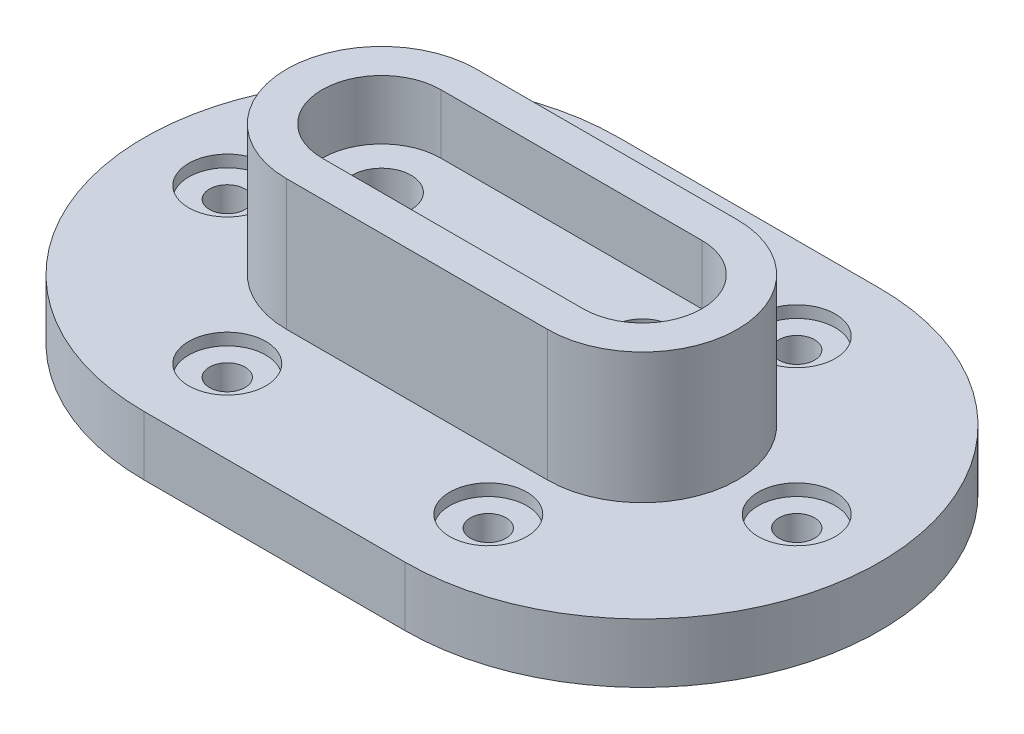
ISO-10303-21;
HEADER;
FILE_DESCRIPTION(('STEP AP214'),'2;1');
FILE_NAME('part.step','',(''),(''),'','','');
FILE_SCHEMA(('AUTOMOTIVE_DESIGN { 1 0 10303 214 1 1 1 1 }'));
ENDSEC;
DATA;
#1=APPLICATION_CONTEXT('core data for automotive mechanical design processes');
#2=APPLICATION_PROTOCOL_DEFINITION('international standard','automotive_design',2000,#1);
#3=PRODUCT_CONTEXT('',#1,'mechanical');
#4=PRODUCT('Part','Part','',(#3));
#5=PRODUCT_RELATED_PRODUCT_CATEGORY('part','',(#4));
#6=PRODUCT_DEFINITION_FORMATION('','',#4);
#7=PRODUCT_DEFINITION_CONTEXT('part definition',#1,'design');
#8=PRODUCT_DEFINITION('design','',#6,#7);
#9=PRODUCT_DEFINITION_SHAPE('','',#8);
#10=(LENGTH_UNIT() NAMED_UNIT(*) SI_UNIT(.MILLI.,.METRE.));
#11=(NAMED_UNIT(*) PLANE_ANGLE_UNIT() SI_UNIT($,.RADIAN.));
#12=(NAMED_UNIT(*) SI_UNIT($,.STERADIAN.) SOLID_ANGLE_UNIT());
#13=UNCERTAINTY_MEASURE_WITH_UNIT(LENGTH_MEASURE(1.E-05),#10,'distance_accuracy_value','');
#14=(GEOMETRIC_REPRESENTATION_CONTEXT(3) GLOBAL_UNCERTAINTY_ASSIGNED_CONTEXT((#13)) GLOBAL_UNIT_ASSIGNED_CONTEXT((#10,
#11,#12)) REPRESENTATION_CONTEXT('',''));
#15=CARTESIAN_POINT('',(0.,0.,0.));
#16=DIRECTION('',(0.,0.,1.));
#17=DIRECTION('',(1.,0.,0.));
#18=AXIS2_PLACEMENT_3D('',#15,#16,#17);
#19=CARTESIAN_POINT('',(-22.,10.,0.));
#20=DIRECTION('',(0.,-1.,0.));
#21=DIRECTION('',(0.,0.,-1.));
#22=AXIS2_PLACEMENT_3D('',#19,#20,#21);
#23=CYLINDRICAL_SURFACE('',#22,40.);
#24=CARTESIAN_POINT('',(-22.,0.,0.));
#25=DIRECTION('',(0.,1.,0.));
#26=DIRECTION('',(0.,0.,1.));
#27=AXIS2_PLACEMENT_3D('',#24,#25,#26);
#28=CIRCLE('',#27,40.);
#29=CARTESIAN_POINT('',(-22.0000000000001,0.,-40.));
#30=VERTEX_POINT('',#29);
#31=CARTESIAN_POINT('',(-21.9999999999996,0.,40.));
#32=VERTEX_POINT('',#31);
#33=EDGE_CURVE('E206',#30,#32,#28,.T.);
#34=ORIENTED_EDGE('',*,*,#33,.T.);
#35=DIRECTION('',(0.,-1.,0.));
#36=VECTOR('',#35,1.);
#37=CARTESIAN_POINT('',(-21.9999999999996,10.,40.));
#38=LINE('',#37,#36);
#39=CARTESIAN_POINT('',(-21.9999999999996,10.,40.));
#40=VERTEX_POINT('',#39);
#41=EDGE_CURVE('E11',#40,#32,#38,.T.);
#42=ORIENTED_EDGE('',*,*,#41,.F.);
#43=CARTESIAN_POINT('',(-22.,10.,0.));
#44=DIRECTION('',(0.,1.,0.));
#45=DIRECTION('',(0.,0.,1.));
#46=AXIS2_PLACEMENT_3D('',#43,#44,#45);
#47=CIRCLE('',#46,40.);
#48=CARTESIAN_POINT('',(-22.0000000000001,10.,-40.));
#49=VERTEX_POINT('',#48);
#50=EDGE_CURVE('E210',#49,#40,#47,.T.);
#51=ORIENTED_EDGE('',*,*,#50,.F.);
#52=DIRECTION('',(0.,-1.,0.));
#53=VECTOR('',#52,1.);
#54=CARTESIAN_POINT('',(-22.0000000000001,10.,-40.));
#55=LINE('',#54,#53);
#56=EDGE_CURVE('E220',#49,#30,#55,.T.);
#57=ORIENTED_EDGE('',*,*,#56,.T.);
#58=EDGE_LOOP('',(#34,#42,#51,#57));
#59=FACE_BOUND('',#58,.T.);
#60=ADVANCED_FACE('F44',(#59),#23,.T.);
#61=CARTESIAN_POINT('',(-21.9999999999996,10.,40.));
#62=DIRECTION('',(0.,0.,-1.));
#63=DIRECTION('',(-1.,0.,0.));
#64=AXIS2_PLACEMENT_3D('',#61,#62,#63);
#65=PLANE('',#64);
#66=DIRECTION('',(1.,0.,0.));
#67=VECTOR('',#66,1.);
#68=CARTESIAN_POINT('',(-21.9999999999996,0.,40.));
#69=LINE('',#68,#67);
#70=CARTESIAN_POINT('',(22.0000000000004,0.,40.));
#71=VERTEX_POINT('',#70);
#72=EDGE_CURVE('E219',#32,#71,#69,.T.);
#73=ORIENTED_EDGE('',*,*,#72,.T.);
#74=DIRECTION('',(0.,-1.,0.));
#75=VECTOR('',#74,1.);
#76=CARTESIAN_POINT('',(22.0000000000004,10.,40.));
#77=LINE('',#76,#75);
#78=CARTESIAN_POINT('',(22.0000000000004,10.,40.));
#79=VERTEX_POINT('',#78);
#80=EDGE_CURVE('E52',#79,#71,#77,.T.);
#81=ORIENTED_EDGE('',*,*,#80,.F.);
#82=DIRECTION('',(1.,0.,0.));
#83=VECTOR('',#82,1.);
#84=CARTESIAN_POINT('',(-21.9999999999996,10.,40.));
#85=LINE('',#84,#83);
#86=EDGE_CURVE('E209',#40,#79,#85,.T.);
#87=ORIENTED_EDGE('',*,*,#86,.F.);
#88=ORIENTED_EDGE('',*,*,#41,.T.);
#89=EDGE_LOOP('',(#73,#81,#87,#88));
#90=FACE_BOUND('',#89,.T.);
#91=ADVANCED_FACE('F318',(#90),#65,.F.);
#92=CARTESIAN_POINT('',(22.,10.,0.));
#93=DIRECTION('',(0.,-1.,0.));
#94=DIRECTION('',(0.,0.,-1.));
#95=AXIS2_PLACEMENT_3D('',#92,#93,#94);
#96=CYLINDRICAL_SURFACE('',#95,40.);
#97=CARTESIAN_POINT('',(22.,0.,0.));
#98=DIRECTION('',(0.,1.,0.));
#99=DIRECTION('',(0.,0.,1.));
#100=AXIS2_PLACEMENT_3D('',#97,#98,#99);
#101=CIRCLE('',#100,40.);
#102=CARTESIAN_POINT('',(21.9999999999999,0.,-40.));
#103=VERTEX_POINT('',#102);
#104=EDGE_CURVE('E225',#71,#103,#101,.T.);
#105=ORIENTED_EDGE('',*,*,#104,.T.);
#106=DIRECTION('',(0.,-1.,0.));
#107=VECTOR('',#106,1.);
#108=CARTESIAN_POINT('',(21.9999999999999,10.,-40.));
#109=LINE('',#108,#107);
#110=CARTESIAN_POINT('',(21.9999999999999,10.,-40.));
#111=VERTEX_POINT('',#110);
#112=EDGE_CURVE('E229',#111,#103,#109,.T.);
#113=ORIENTED_EDGE('',*,*,#112,.F.);
#114=CARTESIAN_POINT('',(22.,10.,0.));
#115=DIRECTION('',(0.,1.,0.));
#116=DIRECTION('',(0.,0.,1.));
#117=AXIS2_PLACEMENT_3D('',#114,#115,#116);
#118=CIRCLE('',#117,40.);
#119=EDGE_CURVE('E213',#79,#111,#118,.T.);
#120=ORIENTED_EDGE('',*,*,#119,.F.);
#121=ORIENTED_EDGE('',*,*,#80,.T.);
#122=EDGE_LOOP('',(#105,#113,#120,#121));
#123=FACE_BOUND('',#122,.T.);
#124=ADVANCED_FACE('F323',(#123),#96,.T.);
#125=CARTESIAN_POINT('',(-22.0000000000001,10.,-40.));
#126=DIRECTION('',(0.,0.,1.));
#127=DIRECTION('',(1.,0.,0.));
#128=AXIS2_PLACEMENT_3D('',#125,#126,#127);
#129=PLANE('',#128);
#130=DIRECTION('',(-1.,0.,0.));
#131=VECTOR('',#130,1.);
#132=CARTESIAN_POINT('',(-22.0000000000001,0.,-40.));
#133=LINE('',#132,#131);
#134=EDGE_CURVE('E211',#103,#30,#133,.T.);
#135=ORIENTED_EDGE('',*,*,#134,.T.);
#136=ORIENTED_EDGE('',*,*,#56,.F.);
#137=DIRECTION('',(-1.,0.,0.));
#138=VECTOR('',#137,1.);
#139=CARTESIAN_POINT('',(-22.0000000000001,10.,-40.));
#140=LINE('',#139,#138);
#141=EDGE_CURVE('E214',#111,#49,#140,.T.);
#142=ORIENTED_EDGE('',*,*,#141,.F.);
#143=ORIENTED_EDGE('',*,*,#112,.T.);
#144=EDGE_LOOP('',(#135,#136,#142,#143));
#145=FACE_BOUND('',#144,.T.);
#146=ADVANCED_FACE('F340',(#145),#129,.F.);
#147=CARTESIAN_POINT('',(-22.,10.,0.));
#148=DIRECTION('',(0.,1.,0.));
#149=DIRECTION('',(0.,0.,1.));
#150=AXIS2_PLACEMENT_3D('',#147,#148,#149);
#151=PLANE('',#150);
#152=CARTESIAN_POINT('',(48.,10.,0.));
#153=DIRECTION('',(0.,1.,0.));
#154=DIRECTION('',(0.,0.,1.));
#155=AXIS2_PLACEMENT_3D('',#152,#153,#154);
#156=CIRCLE('',#155,6.5);
#157=CARTESIAN_POINT('',(48.,10.,6.5));
#158=VERTEX_POINT('',#157);
#159=EDGE_CURVE('E264',#158,#158,#156,.T.);
#160=ORIENTED_EDGE('',*,*,#159,.F.);
#161=EDGE_LOOP('',(#160));
#162=FACE_BOUND('',#161,.T.);
#163=CARTESIAN_POINT('',(22.,10.,26.));
#164=DIRECTION('',(0.,1.,0.));
#165=DIRECTION('',(0.,0.,1.));
#166=AXIS2_PLACEMENT_3D('',#163,#164,#165);
#167=CIRCLE('',#166,6.5);
#168=CARTESIAN_POINT('',(22.,10.,32.5));
#169=VERTEX_POINT('',#168);
#170=EDGE_CURVE('E250',#169,#169,#167,.T.);
#171=ORIENTED_EDGE('',*,*,#170,.F.);
#172=EDGE_LOOP('',(#171));
#173=FACE_BOUND('',#172,.T.);
#174=CARTESIAN_POINT('',(-22.,10.,26.));
#175=DIRECTION('',(0.,1.,0.));
#176=DIRECTION('',(0.,0.,1.));
#177=AXIS2_PLACEMENT_3D('',#174,#175,#176);
#178=CIRCLE('',#177,6.5);
#179=CARTESIAN_POINT('',(-22.,10.,32.5));
#180=VERTEX_POINT('',#179);
#181=EDGE_CURVE('E256',#180,#180,#178,.T.);
#182=ORIENTED_EDGE('',*,*,#181,.F.);
#183=EDGE_LOOP('',(#182));
#184=FACE_BOUND('',#183,.T.);
#185=CARTESIAN_POINT('',(-48.,10.,0.));
#186=DIRECTION('',(0.,1.,0.));
#187=DIRECTION('',(0.,0.,1.));
#188=AXIS2_PLACEMENT_3D('',#185,#186,#187);
#189=CIRCLE('',#188,6.5);
#190=CARTESIAN_POINT('',(-48.,10.,6.5));
#191=VERTEX_POINT('',#190);
#192=EDGE_CURVE('E279',#191,#191,#189,.T.);
#193=ORIENTED_EDGE('',*,*,#192,.F.);
#194=EDGE_LOOP('',(#193));
#195=FACE_BOUND('',#194,.T.);
#196=CARTESIAN_POINT('',(-22.,10.,-26.));
#197=DIRECTION('',(0.,1.,0.));
#198=DIRECTION('',(0.,0.,1.));
#199=AXIS2_PLACEMENT_3D('',#196,#197,#198);
#200=CIRCLE('',#199,6.5);
#201=CARTESIAN_POINT('',(-22.,10.,-19.5));
#202=VERTEX_POINT('',#201);
#203=EDGE_CURVE('E275',#202,#202,#200,.T.);
#204=ORIENTED_EDGE('',*,*,#203,.F.);
#205=EDGE_LOOP('',(#204));
#206=FACE_BOUND('',#205,.T.);
#207=CARTESIAN_POINT('',(22.,10.,-26.));
#208=DIRECTION('',(0.,1.,0.));
#209=DIRECTION('',(0.,0.,1.));
#210=AXIS2_PLACEMENT_3D('',#207,#208,#209);
#211=CIRCLE('',#210,6.5);
#212=CARTESIAN_POINT('',(22.,10.,-19.5));
#213=VERTEX_POINT('',#212);
#214=EDGE_CURVE('E266',#213,#213,#211,.T.);
#215=ORIENTED_EDGE('',*,*,#214,.F.);
#216=EDGE_LOOP('',(#215));
#217=FACE_BOUND('',#216,.T.);
#218=CARTESIAN_POINT('',(-22.,10.,0.));
#219=DIRECTION('',(0.,1.,0.));
#220=DIRECTION('',(0.,0.,1.));
#221=AXIS2_PLACEMENT_3D('',#218,#219,#220);
#222=CIRCLE('',#221,16.);
#223=CARTESIAN_POINT('',(-22.,10.,-16.));
#224=VERTEX_POINT('',#223);
#225=CARTESIAN_POINT('',(-22.,10.,16.));
#226=VERTEX_POINT('',#225);
#227=EDGE_CURVE('E70',#224,#226,#222,.T.);
#228=ORIENTED_EDGE('',*,*,#227,.F.);
#229=DIRECTION('',(-1.,0.,0.));
#230=VECTOR('',#229,1.);
#231=CARTESIAN_POINT('',(-22.,10.,-16.));
#232=LINE('',#231,#230);
#233=CARTESIAN_POINT('',(22.,10.,-16.));
#234=VERTEX_POINT('',#233);
#235=EDGE_CURVE('E176',#234,#224,#232,.T.);
#236=ORIENTED_EDGE('',*,*,#235,.F.);
#237=CARTESIAN_POINT('',(22.,10.,0.));
#238=DIRECTION('',(0.,1.,0.));
#239=DIRECTION('',(0.,0.,1.));
#240=AXIS2_PLACEMENT_3D('',#237,#238,#239);
#241=CIRCLE('',#240,16.);
#242=CARTESIAN_POINT('',(22.,10.,16.));
#243=VERTEX_POINT('',#242);
#244=EDGE_CURVE('E193',#243,#234,#241,.T.);
#245=ORIENTED_EDGE('',*,*,#244,.F.);
#246=DIRECTION('',(1.,0.,0.));
#247=VECTOR('',#246,1.);
#248=CARTESIAN_POINT('',(-22.,10.,16.));
#249=LINE('',#248,#247);
#250=EDGE_CURVE('E187',#226,#243,#249,.T.);
#251=ORIENTED_EDGE('',*,*,#250,.F.);
#252=EDGE_LOOP('',(#228,#236,#245,#251));
#253=FACE_BOUND('',#252,.T.);
#254=ORIENTED_EDGE('',*,*,#50,.T.);
#255=ORIENTED_EDGE('',*,*,#86,.T.);
#256=ORIENTED_EDGE('',*,*,#119,.T.);
#257=ORIENTED_EDGE('',*,*,#141,.T.);
#258=EDGE_LOOP('',(#254,#255,#256,#257));
#259=FACE_BOUND('',#258,.T.);
#260=ADVANCED_FACE('F333',(#162,#173,#184,#195,#206,#217,#253,#259),#151,.T.);
#261=CARTESIAN_POINT('',(-22.,0.,0.));
#262=DIRECTION('',(0.,1.,0.));
#263=DIRECTION('',(0.,0.,1.));
#264=AXIS2_PLACEMENT_3D('',#261,#262,#263);
#265=PLANE('',#264);
#266=CARTESIAN_POINT('',(48.,0.,0.));
#267=DIRECTION('',(0.,1.,0.));
#268=DIRECTION('',(0.,0.,1.));
#269=AXIS2_PLACEMENT_3D('',#266,#267,#268);
#270=CIRCLE('',#269,3.);
#271=CARTESIAN_POINT('',(48.,0.,3.));
#272=VERTEX_POINT('',#271);
#273=EDGE_CURVE('E48',#272,#272,#270,.T.);
#274=ORIENTED_EDGE('',*,*,#273,.T.);
#275=EDGE_LOOP('',(#274));
#276=FACE_BOUND('',#275,.T.);
#277=CARTESIAN_POINT('',(22.,0.,-26.));
#278=DIRECTION('',(0.,1.,0.));
#279=DIRECTION('',(0.,0.,1.));
#280=AXIS2_PLACEMENT_3D('',#277,#278,#279);
#281=CIRCLE('',#280,3.);
#282=CARTESIAN_POINT('',(22.,0.,-23.));
#283=VERTEX_POINT('',#282);
#284=EDGE_CURVE('E245',#283,#283,#281,.T.);
#285=ORIENTED_EDGE('',*,*,#284,.T.);
#286=EDGE_LOOP('',(#285));
#287=FACE_BOUND('',#286,.T.);
#288=CARTESIAN_POINT('',(-22.,0.,-26.));
#289=DIRECTION('',(0.,1.,0.));
#290=DIRECTION('',(0.,0.,1.));
#291=AXIS2_PLACEMENT_3D('',#288,#289,#290);
#292=CIRCLE('',#291,3.);
#293=CARTESIAN_POINT('',(-22.,0.,-23.));
#294=VERTEX_POINT('',#293);
#295=EDGE_CURVE('E244',#294,#294,#292,.T.);
#296=ORIENTED_EDGE('',*,*,#295,.T.);
#297=EDGE_LOOP('',(#296));
#298=FACE_BOUND('',#297,.T.);
#299=CARTESIAN_POINT('',(-48.,0.,0.));
#300=DIRECTION('',(0.,1.,0.));
#301=DIRECTION('',(0.,0.,1.));
#302=AXIS2_PLACEMENT_3D('',#299,#300,#301);
#303=CIRCLE('',#302,3.);
#304=CARTESIAN_POINT('',(-48.,0.,3.));
#305=VERTEX_POINT('',#304);
#306=EDGE_CURVE('E239',#305,#305,#303,.T.);
#307=ORIENTED_EDGE('',*,*,#306,.T.);
#308=EDGE_LOOP('',(#307));
#309=FACE_BOUND('',#308,.T.);
#310=CARTESIAN_POINT('',(-22.,0.,26.));
#311=DIRECTION('',(0.,1.,0.));
#312=DIRECTION('',(0.,0.,1.));
#313=AXIS2_PLACEMENT_3D('',#310,#311,#312);
#314=CIRCLE('',#313,3.);
#315=CARTESIAN_POINT('',(-22.,0.,29.));
#316=VERTEX_POINT('',#315);
#317=EDGE_CURVE('E231',#316,#316,#314,.T.);
#318=ORIENTED_EDGE('',*,*,#317,.T.);
#319=EDGE_LOOP('',(#318));
#320=FACE_BOUND('',#319,.T.);
#321=CARTESIAN_POINT('',(22.,0.,26.));
#322=DIRECTION('',(0.,1.,0.));
#323=DIRECTION('',(0.,0.,1.));
#324=AXIS2_PLACEMENT_3D('',#321,#322,#323);
#325=CIRCLE('',#324,3.);
#326=CARTESIAN_POINT('',(22.,0.,29.));
#327=VERTEX_POINT('',#326);
#328=EDGE_CURVE('E234',#327,#327,#325,.T.);
#329=ORIENTED_EDGE('',*,*,#328,.T.);
#330=EDGE_LOOP('',(#329));
#331=FACE_BOUND('',#330,.T.);
#332=CARTESIAN_POINT('',(22.,0.,0.));
#333=DIRECTION('',(0.,1.,0.));
#334=DIRECTION('',(0.,0.,1.));
#335=AXIS2_PLACEMENT_3D('',#332,#333,#334);
#336=CIRCLE('',#335,5.);
#337=CARTESIAN_POINT('',(22.,0.,5.));
#338=VERTEX_POINT('',#337);
#339=EDGE_CURVE('E161',#338,#338,#336,.T.);
#340=ORIENTED_EDGE('',*,*,#339,.T.);
#341=EDGE_LOOP('',(#340));
#342=FACE_BOUND('',#341,.T.);
#343=CARTESIAN_POINT('',(-22.,0.,0.));
#344=DIRECTION('',(0.,1.,0.));
#345=DIRECTION('',(0.,0.,1.));
#346=AXIS2_PLACEMENT_3D('',#343,#344,#345);
#347=CIRCLE('',#346,5.);
#348=CARTESIAN_POINT('',(-22.,0.,5.));
#349=VERTEX_POINT('',#348);
#350=EDGE_CURVE('E290',#349,#349,#347,.T.);
#351=ORIENTED_EDGE('',*,*,#350,.T.);
#352=EDGE_LOOP('',(#351));
#353=FACE_BOUND('',#352,.T.);
#354=ORIENTED_EDGE('',*,*,#33,.F.);
#355=ORIENTED_EDGE('',*,*,#134,.F.);
#356=ORIENTED_EDGE('',*,*,#104,.F.);
#357=ORIENTED_EDGE('',*,*,#72,.F.);
#358=EDGE_LOOP('',(#354,#355,#356,#357));
#359=FACE_BOUND('',#358,.T.);
#360=ADVANCED_FACE('F300',(#276,#287,#298,#309,#320,#331,#342,#353,#359),#265,.F.);
#361=CARTESIAN_POINT('',(-22.,32.,0.));
#362=DIRECTION('',(0.,-1.,0.));
#363=DIRECTION('',(0.,0.,-1.));
#364=AXIS2_PLACEMENT_3D('',#361,#362,#363);
#365=CYLINDRICAL_SURFACE('',#364,16.);
#366=ORIENTED_EDGE('',*,*,#227,.T.);
#367=DIRECTION('',(0.,-1.,0.));
#368=VECTOR('',#367,1.);
#369=CARTESIAN_POINT('',(-22.,32.,16.));
#370=LINE('',#369,#368);
#371=CARTESIAN_POINT('',(-22.,32.,16.));
#372=VERTEX_POINT('',#371);
#373=EDGE_CURVE('E201',#372,#226,#370,.T.);
#374=ORIENTED_EDGE('',*,*,#373,.F.);
#375=CARTESIAN_POINT('',(-22.,32.,0.));
#376=DIRECTION('',(0.,1.,0.));
#377=DIRECTION('',(0.,0.,1.));
#378=AXIS2_PLACEMENT_3D('',#375,#376,#377);
#379=CIRCLE('',#378,16.);
#380=CARTESIAN_POINT('',(-22.,32.,-16.));
#381=VERTEX_POINT('',#380);
#382=EDGE_CURVE('E178',#381,#372,#379,.T.);
#383=ORIENTED_EDGE('',*,*,#382,.F.);
#384=DIRECTION('',(0.,-1.,0.));
#385=VECTOR('',#384,1.);
#386=CARTESIAN_POINT('',(-22.,32.,-16.));
#387=LINE('',#386,#385);
#388=EDGE_CURVE('E188',#381,#224,#387,.T.);
#389=ORIENTED_EDGE('',*,*,#388,.T.);
#390=EDGE_LOOP('',(#366,#374,#383,#389));
#391=FACE_BOUND('',#390,.T.);
#392=ADVANCED_FACE('F348',(#391),#365,.T.);
#393=CARTESIAN_POINT('',(-22.,32.,16.));
#394=DIRECTION('',(0.,0.,-1.));
#395=DIRECTION('',(-1.,0.,0.));
#396=AXIS2_PLACEMENT_3D('',#393,#394,#395);
#397=PLANE('',#396);
#398=ORIENTED_EDGE('',*,*,#250,.T.);
#399=DIRECTION('',(0.,-1.,0.));
#400=VECTOR('',#399,1.);
#401=CARTESIAN_POINT('',(22.,32.,16.));
#402=LINE('',#401,#400);
#403=CARTESIAN_POINT('',(22.,32.,16.));
#404=VERTEX_POINT('',#403);
#405=EDGE_CURVE('E199',#404,#243,#402,.T.);
#406=ORIENTED_EDGE('',*,*,#405,.F.);
#407=DIRECTION('',(1.,0.,0.));
#408=VECTOR('',#407,1.);
#409=CARTESIAN_POINT('',(-22.,32.,16.));
#410=LINE('',#409,#408);
#411=EDGE_CURVE('E180',#372,#404,#410,.T.);
#412=ORIENTED_EDGE('',*,*,#411,.F.);
#413=ORIENTED_EDGE('',*,*,#373,.T.);
#414=EDGE_LOOP('',(#398,#406,#412,#413));
#415=FACE_BOUND('',#414,.T.);
#416=ADVANCED_FACE('F358',(#415),#397,.F.);
#417=CARTESIAN_POINT('',(22.,32.,0.));
#418=DIRECTION('',(0.,-1.,0.));
#419=DIRECTION('',(0.,0.,-1.));
#420=AXIS2_PLACEMENT_3D('',#417,#418,#419);
#421=CYLINDRICAL_SURFACE('',#420,16.);
#422=ORIENTED_EDGE('',*,*,#244,.T.);
#423=DIRECTION('',(0.,-1.,0.));
#424=VECTOR('',#423,1.);
#425=CARTESIAN_POINT('',(22.,32.,-16.));
#426=LINE('',#425,#424);
#427=CARTESIAN_POINT('',(22.,32.,-16.));
#428=VERTEX_POINT('',#427);
#429=EDGE_CURVE('E197',#428,#234,#426,.T.);
#430=ORIENTED_EDGE('',*,*,#429,.F.);
#431=CARTESIAN_POINT('',(22.,32.,0.));
#432=DIRECTION('',(0.,1.,0.));
#433=DIRECTION('',(0.,0.,1.));
#434=AXIS2_PLACEMENT_3D('',#431,#432,#433);
#435=CIRCLE('',#434,16.);
#436=EDGE_CURVE('E185',#404,#428,#435,.T.);
#437=ORIENTED_EDGE('',*,*,#436,.F.);
#438=ORIENTED_EDGE('',*,*,#405,.T.);
#439=EDGE_LOOP('',(#422,#430,#437,#438));
#440=FACE_BOUND('',#439,.T.);
#441=ADVANCED_FACE('F356',(#440),#421,.T.);
#442=CARTESIAN_POINT('',(-22.,32.,-16.));
#443=DIRECTION('',(0.,0.,1.));
#444=DIRECTION('',(1.,0.,0.));
#445=AXIS2_PLACEMENT_3D('',#442,#443,#444);
#446=PLANE('',#445);
#447=ORIENTED_EDGE('',*,*,#235,.T.);
#448=ORIENTED_EDGE('',*,*,#388,.F.);
#449=DIRECTION('',(-1.,0.,0.));
#450=VECTOR('',#449,1.);
#451=CARTESIAN_POINT('',(-22.,32.,-16.));
#452=LINE('',#451,#450);
#453=EDGE_CURVE('E184',#428,#381,#452,.T.);
#454=ORIENTED_EDGE('',*,*,#453,.F.);
#455=ORIENTED_EDGE('',*,*,#429,.T.);
#456=EDGE_LOOP('',(#447,#448,#454,#455));
#457=FACE_BOUND('',#456,.T.);
#458=ADVANCED_FACE('F365',(#457),#446,.F.);
#459=CARTESIAN_POINT('',(-22.,32.,0.));
#460=DIRECTION('',(0.,1.,0.));
#461=DIRECTION('',(0.,0.,1.));
#462=AXIS2_PLACEMENT_3D('',#459,#460,#461);
#463=PLANE('',#462);
#464=CARTESIAN_POINT('',(-22.,32.,0.));
#465=DIRECTION('',(0.,1.,0.));
#466=DIRECTION('',(0.,0.,1.));
#467=AXIS2_PLACEMENT_3D('',#464,#465,#466);
#468=CIRCLE('',#467,10.);
#469=CARTESIAN_POINT('',(-22.,32.,-10.));
#470=VERTEX_POINT('',#469);
#471=CARTESIAN_POINT('',(-22.,32.,9.99999999999999));
#472=VERTEX_POINT('',#471);
#473=EDGE_CURVE('E63',#470,#472,#468,.T.);
#474=ORIENTED_EDGE('',*,*,#473,.F.);
#475=DIRECTION('',(-1.,0.,0.));
#476=VECTOR('',#475,1.);
#477=CARTESIAN_POINT('',(-22.,32.,-10.));
#478=LINE('',#477,#476);
#479=CARTESIAN_POINT('',(22.,32.,-10.));
#480=VERTEX_POINT('',#479);
#481=EDGE_CURVE('E154',#480,#470,#478,.T.);
#482=ORIENTED_EDGE('',*,*,#481,.F.);
#483=CARTESIAN_POINT('',(22.,32.,0.));
#484=DIRECTION('',(0.,1.,0.));
#485=DIRECTION('',(0.,0.,1.));
#486=AXIS2_PLACEMENT_3D('',#483,#484,#485);
#487=CIRCLE('',#486,10.);
#488=CARTESIAN_POINT('',(22.,32.,10.));
#489=VERTEX_POINT('',#488);
#490=EDGE_CURVE('E158',#489,#480,#487,.T.);
#491=ORIENTED_EDGE('',*,*,#490,.F.);
#492=DIRECTION('',(1.,0.,0.));
#493=VECTOR('',#492,1.);
#494=CARTESIAN_POINT('',(-22.,32.,9.99999999999999));
#495=LINE('',#494,#493);
#496=EDGE_CURVE('E170',#472,#489,#495,.T.);
#497=ORIENTED_EDGE('',*,*,#496,.F.);
#498=EDGE_LOOP('',(#474,#482,#491,#497));
#499=FACE_BOUND('',#498,.T.);
#500=ORIENTED_EDGE('',*,*,#382,.T.);
#501=ORIENTED_EDGE('',*,*,#411,.T.);
#502=ORIENTED_EDGE('',*,*,#436,.T.);
#503=ORIENTED_EDGE('',*,*,#453,.T.);
#504=EDGE_LOOP('',(#500,#501,#502,#503));
#505=FACE_BOUND('',#504,.T.);
#506=ADVANCED_FACE('F366',(#499,#505),#463,.T.);
#507=CARTESIAN_POINT('',(-22.,22.,0.));
#508=DIRECTION('',(0.,1.,0.));
#509=DIRECTION('',(0.,0.,1.));
#510=AXIS2_PLACEMENT_3D('',#507,#508,#509);
#511=CYLINDRICAL_SURFACE('',#510,10.);
#512=ORIENTED_EDGE('',*,*,#473,.T.);
#513=DIRECTION('',(0.,1.,0.));
#514=VECTOR('',#513,1.);
#515=CARTESIAN_POINT('',(-22.,22.,9.99999999999999));
#516=LINE('',#515,#514);
#517=CARTESIAN_POINT('',(-22.,22.,9.99999999999999));
#518=VERTEX_POINT('',#517);
#519=EDGE_CURVE('E132',#518,#472,#516,.T.);
#520=ORIENTED_EDGE('',*,*,#519,.F.);
#521=CARTESIAN_POINT('',(-22.,22.,0.));
#522=DIRECTION('',(0.,1.,0.));
#523=DIRECTION('',(0.,0.,1.));
#524=AXIS2_PLACEMENT_3D('',#521,#522,#523);
#525=CIRCLE('',#524,10.);
#526=CARTESIAN_POINT('',(-22.,22.,-10.));
#527=VERTEX_POINT('',#526);
#528=EDGE_CURVE('E139',#527,#518,#525,.T.);
#529=ORIENTED_EDGE('',*,*,#528,.F.);
#530=DIRECTION('',(0.,1.,0.));
#531=VECTOR('',#530,1.);
#532=CARTESIAN_POINT('',(-22.,22.,-10.));
#533=LINE('',#532,#531);
#534=EDGE_CURVE('E173',#527,#470,#533,.T.);
#535=ORIENTED_EDGE('',*,*,#534,.T.);
#536=EDGE_LOOP('',(#512,#520,#529,#535));
#537=FACE_BOUND('',#536,.T.);
#538=ADVANCED_FACE('F131',(#537),#511,.F.);
#539=CARTESIAN_POINT('',(-22.,22.,-10.));
#540=DIRECTION('',(0.,0.,-1.));
#541=DIRECTION('',(-1.,0.,0.));
#542=AXIS2_PLACEMENT_3D('',#539,#540,#541);
#543=PLANE('',#542);
#544=ORIENTED_EDGE('',*,*,#481,.T.);
#545=ORIENTED_EDGE('',*,*,#534,.F.);
#546=DIRECTION('',(-1.,0.,0.));
#547=VECTOR('',#546,1.);
#548=CARTESIAN_POINT('',(-22.,22.,-10.));
#549=LINE('',#548,#547);
#550=CARTESIAN_POINT('',(22.,22.,-10.));
#551=VERTEX_POINT('',#550);
#552=EDGE_CURVE('E141',#551,#527,#549,.T.);
#553=ORIENTED_EDGE('',*,*,#552,.F.);
#554=DIRECTION('',(0.,1.,0.));
#555=VECTOR('',#554,1.);
#556=CARTESIAN_POINT('',(22.,22.,-10.));
#557=LINE('',#556,#555);
#558=EDGE_CURVE('E172',#551,#480,#557,.T.);
#559=ORIENTED_EDGE('',*,*,#558,.T.);
#560=EDGE_LOOP('',(#544,#545,#553,#559));
#561=FACE_BOUND('',#560,.T.);
#562=ADVANCED_FACE('F374',(#561),#543,.F.);
#563=CARTESIAN_POINT('',(22.,22.,0.));
#564=DIRECTION('',(0.,1.,0.));
#565=DIRECTION('',(0.,0.,1.));
#566=AXIS2_PLACEMENT_3D('',#563,#564,#565);
#567=CYLINDRICAL_SURFACE('',#566,10.);
#568=ORIENTED_EDGE('',*,*,#490,.T.);
#569=ORIENTED_EDGE('',*,*,#558,.F.);
#570=CARTESIAN_POINT('',(22.,22.,0.));
#571=DIRECTION('',(0.,1.,0.));
#572=DIRECTION('',(0.,0.,1.));
#573=AXIS2_PLACEMENT_3D('',#570,#571,#572);
#574=CIRCLE('',#573,10.);
#575=CARTESIAN_POINT('',(22.,22.,10.));
#576=VERTEX_POINT('',#575);
#577=EDGE_CURVE('E151',#576,#551,#574,.T.);
#578=ORIENTED_EDGE('',*,*,#577,.F.);
#579=DIRECTION('',(0.,1.,0.));
#580=VECTOR('',#579,1.);
#581=CARTESIAN_POINT('',(22.,22.,10.));
#582=LINE('',#581,#580);
#583=EDGE_CURVE('E142',#576,#489,#582,.T.);
#584=ORIENTED_EDGE('',*,*,#583,.T.);
#585=EDGE_LOOP('',(#568,#569,#578,#584));
#586=FACE_BOUND('',#585,.T.);
#587=ADVANCED_FACE('F378',(#586),#567,.F.);
#588=CARTESIAN_POINT('',(-22.,22.,9.99999999999999));
#589=DIRECTION('',(0.,0.,1.));
#590=DIRECTION('',(1.,0.,0.));
#591=AXIS2_PLACEMENT_3D('',#588,#589,#590);
#592=PLANE('',#591);
#593=ORIENTED_EDGE('',*,*,#496,.T.);
#594=ORIENTED_EDGE('',*,*,#583,.F.);
#595=DIRECTION('',(1.,0.,0.));
#596=VECTOR('',#595,1.);
#597=CARTESIAN_POINT('',(-22.,22.,9.99999999999999));
#598=LINE('',#597,#596);
#599=EDGE_CURVE('E148',#518,#576,#598,.T.);
#600=ORIENTED_EDGE('',*,*,#599,.F.);
#601=ORIENTED_EDGE('',*,*,#519,.T.);
#602=EDGE_LOOP('',(#593,#594,#600,#601));
#603=FACE_BOUND('',#602,.T.);
#604=ADVANCED_FACE('F150',(#603),#592,.F.);
#605=CARTESIAN_POINT('',(-22.,22.,0.));
#606=DIRECTION('',(0.,1.,0.));
#607=DIRECTION('',(0.,0.,1.));
#608=AXIS2_PLACEMENT_3D('',#605,#606,#607);
#609=PLANE('',#608);
#610=CARTESIAN_POINT('',(22.,22.,0.));
#611=DIRECTION('',(0.,1.,0.));
#612=DIRECTION('',(0.,0.,1.));
#613=AXIS2_PLACEMENT_3D('',#610,#611,#612);
#614=CIRCLE('',#613,5.);
#615=CARTESIAN_POINT('',(22.,22.,5.));
#616=VERTEX_POINT('',#615);
#617=EDGE_CURVE('E288',#616,#616,#614,.T.);
#618=ORIENTED_EDGE('',*,*,#617,.F.);
#619=EDGE_LOOP('',(#618));
#620=FACE_BOUND('',#619,.T.);
#621=CARTESIAN_POINT('',(-22.,22.,0.));
#622=DIRECTION('',(0.,1.,0.));
#623=DIRECTION('',(0.,0.,1.));
#624=AXIS2_PLACEMENT_3D('',#621,#622,#623);
#625=CIRCLE('',#624,5.);
#626=CARTESIAN_POINT('',(-22.,22.,5.));
#627=VERTEX_POINT('',#626);
#628=EDGE_CURVE('E286',#627,#627,#625,.T.);
#629=ORIENTED_EDGE('',*,*,#628,.F.);
#630=EDGE_LOOP('',(#629));
#631=FACE_BOUND('',#630,.T.);
#632=ORIENTED_EDGE('',*,*,#528,.T.);
#633=ORIENTED_EDGE('',*,*,#599,.T.);
#634=ORIENTED_EDGE('',*,*,#577,.T.);
#635=ORIENTED_EDGE('',*,*,#552,.T.);
#636=EDGE_LOOP('',(#632,#633,#634,#635));
#637=FACE_BOUND('',#636,.T.);
#638=ADVANCED_FACE('F153',(#620,#631,#637),#609,.T.);
#639=CARTESIAN_POINT('',(-22.,-31.,0.));
#640=DIRECTION('',(0.,1.,0.));
#641=DIRECTION('',(0.,0.,1.));
#642=AXIS2_PLACEMENT_3D('',#639,#640,#641);
#643=CYLINDRICAL_SURFACE('',#642,5.);
#644=ORIENTED_EDGE('',*,*,#628,.T.);
#645=EDGE_LOOP('',(#644));
#646=FACE_BOUND('',#645,.T.);
#647=ORIENTED_EDGE('',*,*,#350,.F.);
#648=EDGE_LOOP('',(#647));
#649=FACE_BOUND('',#648,.T.);
#650=ADVANCED_FACE('F305',(#646,#649),#643,.F.);
#651=CARTESIAN_POINT('',(22.,-31.,0.));
#652=DIRECTION('',(0.,1.,0.));
#653=DIRECTION('',(0.,0.,1.));
#654=AXIS2_PLACEMENT_3D('',#651,#652,#653);
#655=CYLINDRICAL_SURFACE('',#654,5.);
#656=ORIENTED_EDGE('',*,*,#617,.T.);
#657=EDGE_LOOP('',(#656));
#658=FACE_BOUND('',#657,.T.);
#659=ORIENTED_EDGE('',*,*,#339,.F.);
#660=EDGE_LOOP('',(#659));
#661=FACE_BOUND('',#660,.T.);
#662=ADVANCED_FACE('F303',(#658,#661),#655,.F.);
#663=CARTESIAN_POINT('',(22.,8.,-26.));
#664=DIRECTION('',(0.,1.,0.));
#665=DIRECTION('',(0.,0.,1.));
#666=AXIS2_PLACEMENT_3D('',#663,#664,#665);
#667=CYLINDRICAL_SURFACE('',#666,6.5);
#668=CARTESIAN_POINT('',(22.,8.,-26.));
#669=DIRECTION('',(0.,1.,0.));
#670=DIRECTION('',(0.,0.,1.));
#671=AXIS2_PLACEMENT_3D('',#668,#669,#670);
#672=CIRCLE('',#671,6.5);
#673=CARTESIAN_POINT('',(22.,8.,-19.5));
#674=VERTEX_POINT('',#673);
#675=EDGE_CURVE('E265',#674,#674,#672,.T.);
#676=ORIENTED_EDGE('',*,*,#675,.F.);
#677=EDGE_LOOP('',(#676));
#678=FACE_BOUND('',#677,.T.);
#679=ORIENTED_EDGE('',*,*,#214,.T.);
#680=EDGE_LOOP('',(#679));
#681=FACE_BOUND('',#680,.T.);
#682=ADVANCED_FACE('F302',(#678,#681),#667,.F.);
#683=CARTESIAN_POINT('',(22.,8.,-26.));
#684=DIRECTION('',(0.,1.,0.));
#685=DIRECTION('',(0.,0.,1.));
#686=AXIS2_PLACEMENT_3D('',#683,#684,#685);
#687=PLANE('',#686);
#688=CARTESIAN_POINT('',(22.,8.,-26.));
#689=DIRECTION('',(0.,1.,0.));
#690=DIRECTION('',(0.,0.,1.));
#691=AXIS2_PLACEMENT_3D('',#688,#689,#690);
#692=CIRCLE('',#691,3.);
#693=CARTESIAN_POINT('',(22.,8.,-23.));
#694=VERTEX_POINT('',#693);
#695=EDGE_CURVE('E894',#694,#694,#692,.T.);
#696=ORIENTED_EDGE('',*,*,#695,.F.);
#697=EDGE_LOOP('',(#696));
#698=FACE_BOUND('',#697,.T.);
#699=ORIENTED_EDGE('',*,*,#675,.T.);
#700=EDGE_LOOP('',(#699));
#701=FACE_BOUND('',#700,.T.);
#702=ADVANCED_FACE('F313',(#698,#701),#687,.T.);
#703=CARTESIAN_POINT('',(-22.,8.,-26.));
#704=DIRECTION('',(0.,1.,0.));
#705=DIRECTION('',(0.,0.,1.));
#706=AXIS2_PLACEMENT_3D('',#703,#704,#705);
#707=CYLINDRICAL_SURFACE('',#706,6.5);
#708=CARTESIAN_POINT('',(-22.,8.,-26.));
#709=DIRECTION('',(0.,1.,0.));
#710=DIRECTION('',(0.,0.,1.));
#711=AXIS2_PLACEMENT_3D('',#708,#709,#710);
#712=CIRCLE('',#711,6.5);
#713=CARTESIAN_POINT('',(-22.,8.,-19.5));
#714=VERTEX_POINT('',#713);
#715=EDGE_CURVE('E267',#714,#714,#712,.T.);
#716=ORIENTED_EDGE('',*,*,#715,.F.);
#717=EDGE_LOOP('',(#716));
#718=FACE_BOUND('',#717,.T.);
#719=ORIENTED_EDGE('',*,*,#203,.T.);
#720=EDGE_LOOP('',(#719));
#721=FACE_BOUND('',#720,.T.);
#722=ADVANCED_FACE('F423',(#718,#721),#707,.F.);
#723=CARTESIAN_POINT('',(-22.,8.,-26.));
#724=DIRECTION('',(0.,1.,0.));
#725=DIRECTION('',(0.,0.,1.));
#726=AXIS2_PLACEMENT_3D('',#723,#724,#725);
#727=PLANE('',#726);
#728=CARTESIAN_POINT('',(-22.,8.,-26.));
#729=DIRECTION('',(0.,1.,0.));
#730=DIRECTION('',(0.,0.,1.));
#731=AXIS2_PLACEMENT_3D('',#728,#729,#730);
#732=CIRCLE('',#731,3.);
#733=CARTESIAN_POINT('',(-22.,8.,-23.));
#734=VERTEX_POINT('',#733);
#735=EDGE_CURVE('E895',#734,#734,#732,.T.);
#736=ORIENTED_EDGE('',*,*,#735,.F.);
#737=EDGE_LOOP('',(#736));
#738=FACE_BOUND('',#737,.T.);
#739=ORIENTED_EDGE('',*,*,#715,.T.);
#740=EDGE_LOOP('',(#739));
#741=FACE_BOUND('',#740,.T.);
#742=ADVANCED_FACE('F435',(#738,#741),#727,.T.);
#743=CARTESIAN_POINT('',(-48.,8.,0.));
#744=DIRECTION('',(0.,1.,0.));
#745=DIRECTION('',(0.,0.,1.));
#746=AXIS2_PLACEMENT_3D('',#743,#744,#745);
#747=CYLINDRICAL_SURFACE('',#746,6.5);
#748=CARTESIAN_POINT('',(-48.,8.,0.));
#749=DIRECTION('',(0.,1.,0.));
#750=DIRECTION('',(0.,0.,1.));
#751=AXIS2_PLACEMENT_3D('',#748,#749,#750);
#752=CIRCLE('',#751,6.5);
#753=CARTESIAN_POINT('',(-48.,8.,6.5));
#754=VERTEX_POINT('',#753);
#755=EDGE_CURVE('E274',#754,#754,#752,.T.);
#756=ORIENTED_EDGE('',*,*,#755,.F.);
#757=EDGE_LOOP('',(#756));
#758=FACE_BOUND('',#757,.T.);
#759=ORIENTED_EDGE('',*,*,#192,.T.);
#760=EDGE_LOOP('',(#759));
#761=FACE_BOUND('',#760,.T.);
#762=ADVANCED_FACE('F445',(#758,#761),#747,.F.);
#763=CARTESIAN_POINT('',(-48.,8.,0.));
#764=DIRECTION('',(0.,1.,0.));
#765=DIRECTION('',(0.,0.,1.));
#766=AXIS2_PLACEMENT_3D('',#763,#764,#765);
#767=PLANE('',#766);
#768=CARTESIAN_POINT('',(-48.,8.,0.));
#769=DIRECTION('',(0.,1.,0.));
#770=DIRECTION('',(0.,0.,1.));
#771=AXIS2_PLACEMENT_3D('',#768,#769,#770);
#772=CIRCLE('',#771,3.);
#773=CARTESIAN_POINT('',(-48.,8.,3.));
#774=VERTEX_POINT('',#773);
#775=EDGE_CURVE('E896',#774,#774,#772,.T.);
#776=ORIENTED_EDGE('',*,*,#775,.F.);
#777=EDGE_LOOP('',(#776));
#778=FACE_BOUND('',#777,.T.);
#779=ORIENTED_EDGE('',*,*,#755,.T.);
#780=EDGE_LOOP('',(#779));
#781=FACE_BOUND('',#780,.T.);
#782=ADVANCED_FACE('F452',(#778,#781),#767,.T.);
#783=CARTESIAN_POINT('',(-22.,8.,26.));
#784=DIRECTION('',(0.,1.,0.));
#785=DIRECTION('',(0.,0.,1.));
#786=AXIS2_PLACEMENT_3D('',#783,#784,#785);
#787=CYLINDRICAL_SURFACE('',#786,6.5);
#788=CARTESIAN_POINT('',(-22.,8.,26.));
#789=DIRECTION('',(0.,1.,0.));
#790=DIRECTION('',(0.,0.,1.));
#791=AXIS2_PLACEMENT_3D('',#788,#789,#790);
#792=CIRCLE('',#791,6.5);
#793=CARTESIAN_POINT('',(-22.,8.,32.5));
#794=VERTEX_POINT('',#793);
#795=EDGE_CURVE('E283',#794,#794,#792,.T.);
#796=ORIENTED_EDGE('',*,*,#795,.F.);
#797=EDGE_LOOP('',(#796));
#798=FACE_BOUND('',#797,.T.);
#799=ORIENTED_EDGE('',*,*,#181,.T.);
#800=EDGE_LOOP('',(#799));
#801=FACE_BOUND('',#800,.T.);
#802=ADVANCED_FACE('F462',(#798,#801),#787,.F.);
#803=CARTESIAN_POINT('',(-22.,8.,26.));
#804=DIRECTION('',(0.,1.,0.));
#805=DIRECTION('',(0.,0.,1.));
#806=AXIS2_PLACEMENT_3D('',#803,#804,#805);
#807=PLANE('',#806);
#808=CARTESIAN_POINT('',(-22.,8.,26.));
#809=DIRECTION('',(0.,1.,0.));
#810=DIRECTION('',(0.,0.,1.));
#811=AXIS2_PLACEMENT_3D('',#808,#809,#810);
#812=CIRCLE('',#811,3.);
#813=CARTESIAN_POINT('',(-22.,8.,29.));
#814=VERTEX_POINT('',#813);
#815=EDGE_CURVE('E890',#814,#814,#812,.T.);
#816=ORIENTED_EDGE('',*,*,#815,.F.);
#817=EDGE_LOOP('',(#816));
#818=FACE_BOUND('',#817,.T.);
#819=ORIENTED_EDGE('',*,*,#795,.T.);
#820=EDGE_LOOP('',(#819));
#821=FACE_BOUND('',#820,.T.);
#822=ADVANCED_FACE('F471',(#818,#821),#807,.T.);
#823=CARTESIAN_POINT('',(22.,8.,26.));
#824=DIRECTION('',(0.,1.,0.));
#825=DIRECTION('',(0.,0.,1.));
#826=AXIS2_PLACEMENT_3D('',#823,#824,#825);
#827=CYLINDRICAL_SURFACE('',#826,6.5);
#828=CARTESIAN_POINT('',(22.,8.,26.));
#829=DIRECTION('',(0.,1.,0.));
#830=DIRECTION('',(0.,0.,1.));
#831=AXIS2_PLACEMENT_3D('',#828,#829,#830);
#832=CIRCLE('',#831,6.5);
#833=CARTESIAN_POINT('',(22.,8.,32.5));
#834=VERTEX_POINT('',#833);
#835=EDGE_CURVE('E251',#834,#834,#832,.T.);
#836=ORIENTED_EDGE('',*,*,#835,.F.);
#837=EDGE_LOOP('',(#836));
#838=FACE_BOUND('',#837,.T.);
#839=ORIENTED_EDGE('',*,*,#170,.T.);
#840=EDGE_LOOP('',(#839));
#841=FACE_BOUND('',#840,.T.);
#842=ADVANCED_FACE('F485',(#838,#841),#827,.F.);
#843=CARTESIAN_POINT('',(22.,8.,26.));
#844=DIRECTION('',(0.,1.,0.));
#845=DIRECTION('',(0.,0.,1.));
#846=AXIS2_PLACEMENT_3D('',#843,#844,#845);
#847=PLANE('',#846);
#848=CARTESIAN_POINT('',(22.,8.,26.));
#849=DIRECTION('',(0.,1.,0.));
#850=DIRECTION('',(0.,0.,1.));
#851=AXIS2_PLACEMENT_3D('',#848,#849,#850);
#852=CIRCLE('',#851,3.);
#853=CARTESIAN_POINT('',(22.,8.,29.));
#854=VERTEX_POINT('',#853);
#855=EDGE_CURVE('E888',#854,#854,#852,.T.);
#856=ORIENTED_EDGE('',*,*,#855,.F.);
#857=EDGE_LOOP('',(#856));
#858=FACE_BOUND('',#857,.T.);
#859=ORIENTED_EDGE('',*,*,#835,.T.);
#860=EDGE_LOOP('',(#859));
#861=FACE_BOUND('',#860,.T.);
#862=ADVANCED_FACE('F495',(#858,#861),#847,.T.);
#863=CARTESIAN_POINT('',(48.,8.,0.));
#864=DIRECTION('',(0.,1.,0.));
#865=DIRECTION('',(0.,0.,1.));
#866=AXIS2_PLACEMENT_3D('',#863,#864,#865);
#867=CYLINDRICAL_SURFACE('',#866,6.5);
#868=CARTESIAN_POINT('',(48.,8.,0.));
#869=DIRECTION('',(0.,1.,0.));
#870=DIRECTION('',(0.,0.,1.));
#871=AXIS2_PLACEMENT_3D('',#868,#869,#870);
#872=CIRCLE('',#871,6.5);
#873=CARTESIAN_POINT('',(48.,8.,6.5));
#874=VERTEX_POINT('',#873);
#875=EDGE_CURVE('E295',#874,#874,#872,.T.);
#876=ORIENTED_EDGE('',*,*,#875,.F.);
#877=EDGE_LOOP('',(#876));
#878=FACE_BOUND('',#877,.T.);
#879=ORIENTED_EDGE('',*,*,#159,.T.);
#880=EDGE_LOOP('',(#879));
#881=FACE_BOUND('',#880,.T.);
#882=ADVANCED_FACE('F503',(#878,#881),#867,.F.);
#883=CARTESIAN_POINT('',(48.,8.,0.));
#884=DIRECTION('',(0.,1.,0.));
#885=DIRECTION('',(0.,0.,1.));
#886=AXIS2_PLACEMENT_3D('',#883,#884,#885);
#887=PLANE('',#886);
#888=CARTESIAN_POINT('',(48.,8.,0.));
#889=DIRECTION('',(0.,1.,0.));
#890=DIRECTION('',(0.,0.,1.));
#891=AXIS2_PLACEMENT_3D('',#888,#889,#890);
#892=CIRCLE('',#891,3.);
#893=CARTESIAN_POINT('',(48.,8.,3.));
#894=VERTEX_POINT('',#893);
#895=EDGE_CURVE('E237',#894,#894,#892,.T.);
#896=ORIENTED_EDGE('',*,*,#895,.F.);
#897=EDGE_LOOP('',(#896));
#898=FACE_BOUND('',#897,.T.);
#899=ORIENTED_EDGE('',*,*,#875,.T.);
#900=EDGE_LOOP('',(#899));
#901=FACE_BOUND('',#900,.T.);
#902=ADVANCED_FACE('F506',(#898,#901),#887,.T.);
#903=CARTESIAN_POINT('',(22.,-32.,26.));
#904=DIRECTION('',(0.,1.,0.));
#905=DIRECTION('',(0.,0.,1.));
#906=AXIS2_PLACEMENT_3D('',#903,#904,#905);
#907=CYLINDRICAL_SURFACE('',#906,3.);
#908=ORIENTED_EDGE('',*,*,#855,.T.);
#909=EDGE_LOOP('',(#908));
#910=FACE_BOUND('',#909,.T.);
#911=ORIENTED_EDGE('',*,*,#328,.F.);
#912=EDGE_LOOP('',(#911));
#913=FACE_BOUND('',#912,.T.);
#914=ADVANCED_FACE('F520',(#910,#913),#907,.F.);
#915=CARTESIAN_POINT('',(-22.,-32.,26.));
#916=DIRECTION('',(0.,1.,0.));
#917=DIRECTION('',(0.,0.,1.));
#918=AXIS2_PLACEMENT_3D('',#915,#916,#917);
#919=CYLINDRICAL_SURFACE('',#918,3.);
#920=ORIENTED_EDGE('',*,*,#815,.T.);
#921=EDGE_LOOP('',(#920));
#922=FACE_BOUND('',#921,.T.);
#923=ORIENTED_EDGE('',*,*,#317,.F.);
#924=EDGE_LOOP('',(#923));
#925=FACE_BOUND('',#924,.T.);
#926=ADVANCED_FACE('F529',(#922,#925),#919,.F.);
#927=CARTESIAN_POINT('',(-48.,-32.,0.));
#928=DIRECTION('',(0.,1.,0.));
#929=DIRECTION('',(0.,0.,1.));
#930=AXIS2_PLACEMENT_3D('',#927,#928,#929);
#931=CYLINDRICAL_SURFACE('',#930,3.);
#932=ORIENTED_EDGE('',*,*,#775,.T.);
#933=EDGE_LOOP('',(#932));
#934=FACE_BOUND('',#933,.T.);
#935=ORIENTED_EDGE('',*,*,#306,.F.);
#936=EDGE_LOOP('',(#935));
#937=FACE_BOUND('',#936,.T.);
#938=ADVANCED_FACE('F541',(#934,#937),#931,.F.);
#939=CARTESIAN_POINT('',(-22.,-32.,-26.));
#940=DIRECTION('',(0.,1.,0.));
#941=DIRECTION('',(0.,0.,1.));
#942=AXIS2_PLACEMENT_3D('',#939,#940,#941);
#943=CYLINDRICAL_SURFACE('',#942,3.);
#944=ORIENTED_EDGE('',*,*,#735,.T.);
#945=EDGE_LOOP('',(#944));
#946=FACE_BOUND('',#945,.T.);
#947=ORIENTED_EDGE('',*,*,#295,.F.);
#948=EDGE_LOOP('',(#947));
#949=FACE_BOUND('',#948,.T.);
#950=ADVANCED_FACE('F552',(#946,#949),#943,.F.);
#951=CARTESIAN_POINT('',(22.,-32.,-26.));
#952=DIRECTION('',(0.,1.,0.));
#953=DIRECTION('',(0.,0.,1.));
#954=AXIS2_PLACEMENT_3D('',#951,#952,#953);
#955=CYLINDRICAL_SURFACE('',#954,3.);
#956=ORIENTED_EDGE('',*,*,#695,.T.);
#957=EDGE_LOOP('',(#956));
#958=FACE_BOUND('',#957,.T.);
#959=ORIENTED_EDGE('',*,*,#284,.F.);
#960=EDGE_LOOP('',(#959));
#961=FACE_BOUND('',#960,.T.);
#962=ADVANCED_FACE('F563',(#958,#961),#955,.F.);
#963=CARTESIAN_POINT('',(48.,-32.,0.));
#964=DIRECTION('',(0.,1.,0.));
#965=DIRECTION('',(0.,0.,1.));
#966=AXIS2_PLACEMENT_3D('',#963,#964,#965);
#967=CYLINDRICAL_SURFACE('',#966,3.);
#968=ORIENTED_EDGE('',*,*,#895,.T.);
#969=EDGE_LOOP('',(#968));
#970=FACE_BOUND('',#969,.T.);
#971=ORIENTED_EDGE('',*,*,#273,.F.);
#972=EDGE_LOOP('',(#971));
#973=FACE_BOUND('',#972,.T.);
#974=ADVANCED_FACE('F573',(#970,#973),#967,.F.);
#975=CLOSED_SHELL('',(#60,#91,#124,#146,#260,#360,#392,#416,#441,#458,#506,#538,#562,#587,#604,
#638,#650,#662,#682,#702,#722,#742,#762,#782,#802,#822,#842,#862,#882,#902,#914,#926,#938,#950,
#962,#974));
#976=MANIFOLD_SOLID_BREP('B2',#975);
#977=ADVANCED_BREP_SHAPE_REPRESENTATION('',(#18,#976),#14);
#978=SHAPE_DEFINITION_REPRESENTATION(#9,#977);
ENDSEC;
END-ISO-10303-21;
